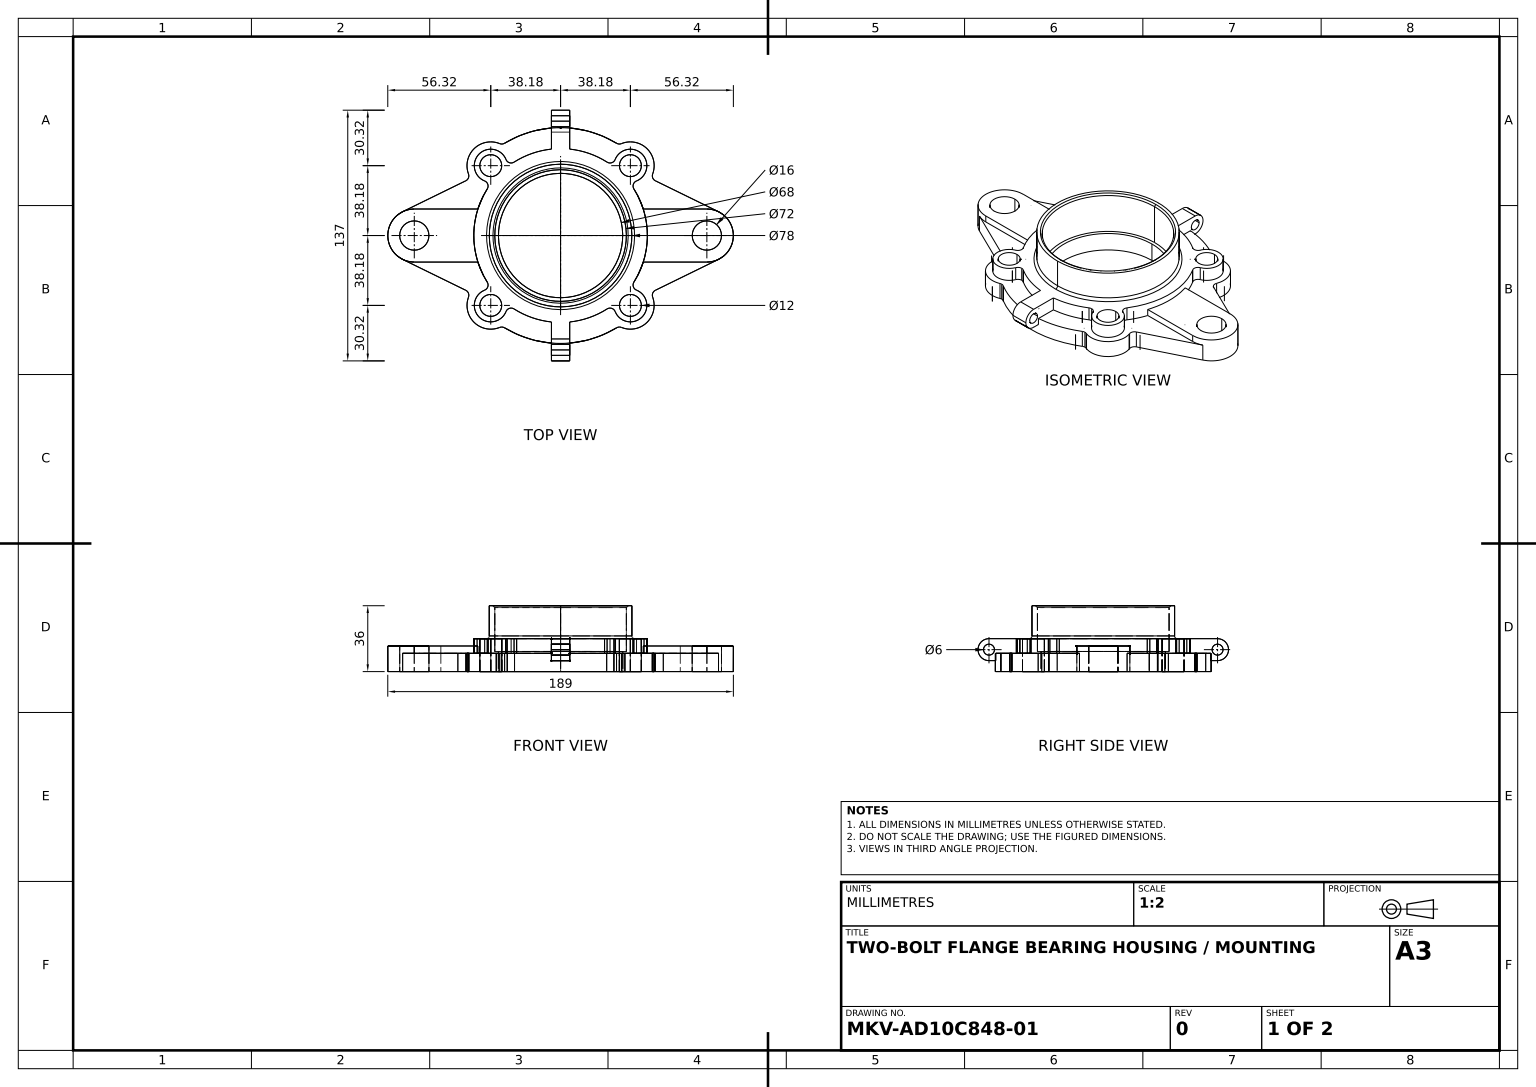
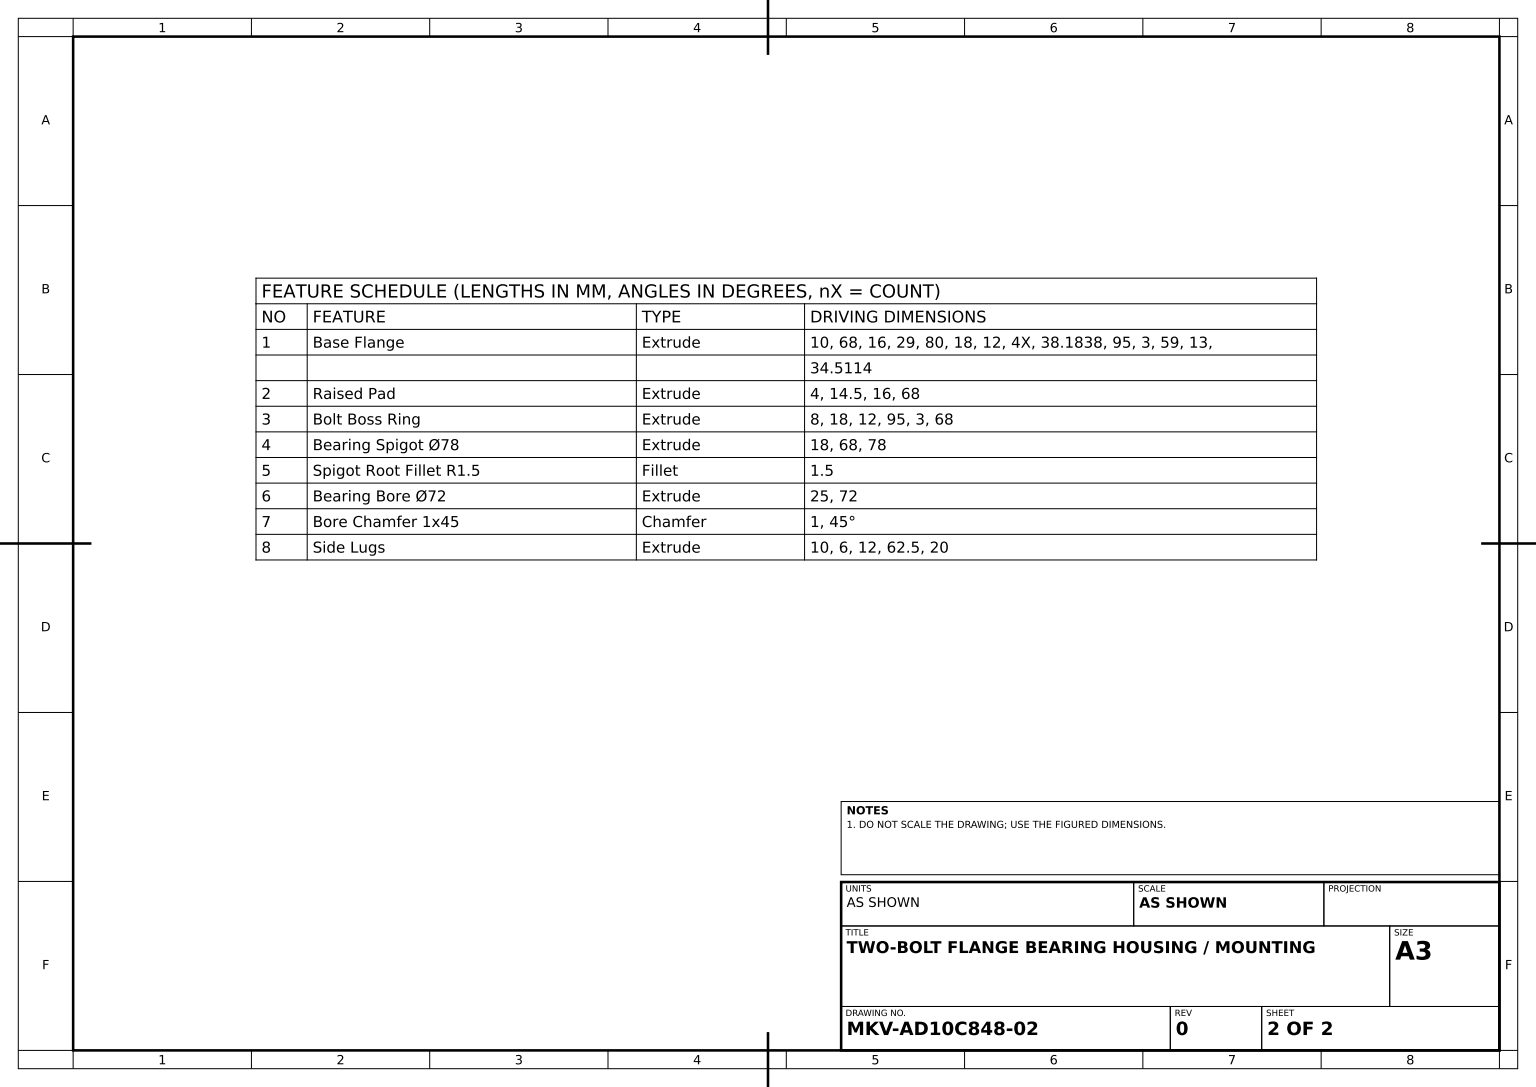
SolidWorks part; units mm, degrees
material "Plain Carbon Steel"
ref_plane "Front Plane" through (0, 0, 0) normal (0, 0, 1) x (1, 0, 0)
ref_plane "Top Plane" through (0, 0, 0) normal (0, 1, 0) x (1, 0, 0)
ref_plane "Right Plane" through (0, 0, 0) normal (1, 0, 0) x (0, 0, -1)
sketch "Base Flange Sketch" plane through (0, 0, 0) normal (0, 1, 0) x (1, 0, 0)
  line L0 (-86.3725, 13.0246) -> (-51.8611, 29.9099)
  line L1 (-86.3725, -13.0246) -> (-51.8611, -29.9099)
  line L2 (86.3725, 13.0246) -> (51.8611, 29.9099)
  line L3 (86.3725, -13.0246) -> (51.8611, -29.9099)
  line L4 (-80, 14.5) -> (-45.2327, 14.5)
  line L5 (-80, -14.5) -> (-45.2327, -14.5)
  line L6 (45.2327, 14.5) -> (80, 14.5)
  line L7 (45.2327, -14.5) -> (80, -14.5)
  circle A0 centre (0, 0) radius 34
  circle A4 centre (-80, 0) radius 8
  arc A5 (-80, 14.5) -> (-80, -14.5) centre (-80, 0) ccw
  arc A6 (80, -14.5) -> (80, 14.5) centre (80, 0) ccw
  circle A7 centre (80, 0) radius 8
  arc A8 (-29.8296, 41.5317) -> (-41.5317, 29.8296) centre (-38.1838, 38.1838) ccw
  circle A10 centre (-38.1838, 38.1838) radius 6
  arc A11 (50.3678, 33.6507) -> (33.2898, 50.2274) centre (38.1838, 38.1838) ccw
  arc A12 (41.5317, 29.8296) -> (29.8296, 41.5317) centre (38.1838, 38.1838) ccw
  circle A13 centre (38.1838, 38.1838) radius 6
  arc A14 (33.2898, -50.2274) -> (50.3678, -33.6507) centre (38.1838, -38.1838) ccw
  arc A15 (29.8296, -41.5317) -> (41.5317, -29.8296) centre (38.1838, -38.1838) ccw
  circle A16 centre (38.1838, -38.1838) radius 6
  arc A17 (-50.3678, -33.6507) -> (-33.2898, -50.2274) centre (-38.1838, -38.1838) ccw
  arc A18 (-41.5317, -29.8296) -> (-29.8296, -41.5317) centre (-38.1838, -38.1838) ccw
  circle A19 centre (-38.1838, -38.1838) radius 6
  arc A20 (-40.1141, 25.4383) -> (-40.1141, -25.4383) centre (0, 0) ccw
  arc A21 (-33.2898, 50.2274) -> (-50.3678, 33.6507) centre (-38.1838, 38.1838) ccw
  arc A22 (-25.4383, -40.1141) -> (25.4383, -40.1141) centre (0, 0) ccw
  arc A23 (-30.6042, -50.4418) -> (30.6042, -50.4418) centre (0, 0) ccw
  arc A24 (25.4383, 40.1141) -> (-25.4383, 40.1141) centre (0, 0) ccw
  arc A25 (30.6042, 50.4418) -> (-30.6042, 50.4418) centre (0, 0) ccw
  arc A26 (40.1141, -25.4383) -> (40.1141, 25.4383) centre (0, 0) ccw
  arc A28 (-30.6042, -50.4418) -> (-33.2898, -50.2274) centre (-32.1604, -53.0067) ccw
  arc A29 (-51.8611, -29.9099) -> (-50.3678, -33.6507) centre (-53.1795, -32.6046) cw
  arc A30 (33.2898, -50.2274) -> (30.6042, -50.4418) centre (32.1604, -53.0067) ccw
  arc A31 (50.3678, -33.6507) -> (51.8611, -29.9099) centre (53.1795, -32.6046) cw
  arc A32 (51.8611, 29.9099) -> (50.3678, 33.6507) centre (53.1795, 32.6046) cw
  arc A33 (33.2898, 50.2274) -> (30.6042, 50.4418) centre (32.1604, 53.0067) cw
  arc A34 (-51.8611, 29.9099) -> (-50.3678, 33.6507) centre (-53.1795, 32.6046) ccw
  arc A35 (-30.6042, 50.4418) -> (-33.2898, 50.2274) centre (-32.1604, 53.0067) cw
  arc A36 (29.8296, -41.5317) -> (25.4383, -40.1141) centre (27.0449, -42.6476) ccw
  arc A37 (41.5317, -29.8296) -> (40.1141, -25.4383) centre (42.6476, -27.0449) cw
  arc A38 (41.5317, 29.8296) -> (40.1141, 25.4383) centre (42.6476, 27.0449) ccw
  arc A39 (29.8296, 41.5317) -> (25.4383, 40.1141) centre (27.0449, 42.6476) cw
  arc A40 (-41.5317, 29.8296) -> (-40.1141, 25.4383) centre (-42.6476, 27.0449) cw
  arc A41 (-41.5317, -29.8296) -> (-40.1141, -25.4383) centre (-42.6476, -27.0449) ccw
  arc A42 (-29.8296, 41.5317) -> (-25.4383, 40.1141) centre (-27.0449, 42.6476) ccw
  arc A43 (-29.8296, -41.5317) -> (-25.4383, -40.1141) centre (-27.0449, -42.6476) cw
  point P41 (49.5957, -31.9573)
  point P46 (31.9573, 49.5957)
  point P55 (37.4544, -29.2134)
  point P60 (29.2134, 37.4544)
  dimension "D1" = 68
  dimension "D3" = 95
  dimension "D4" = 16
  dimension "D5" = 29
  dimension "D6" = 29
  dimension "D7" = 16
  dimension "D8" = 38.1838
  dimension "D11" = 3
  dimension "D12" = 18
  dimension "D13" = 12
  dimension "D20" = 3
  dimension "D21" = 3
  dimension "D22" = 3
  dimension "D23" = 59
  dimension "D24" = 13
  dimension "D25" = 13
  dimension "D26" = 13
  dimension "D27" = 13
  dimension "D9" = 80
  dimension "D10" = 80
  dimension "D15" = 38.1838
  dimension "D16" = 38.1838
  dimension "D17" = 38.1838
  dimension "D18" = 38.1838
  dimension "D19" = 38.1838
  dimension "D28" = 34.5114
  dimension "D29" = 34.5114
  dimension "D30" = 34.5114
  dimension "D31" = 34.5114
  dimension "D14" = 4
extrude "Base Flange" add sketch "Base Flange Sketch" along normal blind 10 contours A20 L4 A5 L5 A4 | A43 A18 A41 A20 L5 A5 L1 A29 A17 A28 A23 A30 A14 A31 L3 A6 L7 A26 A37 A15 A36 A22 | A8 A42 A24 A39 A12 A38 A26 L6 A6 L2 A32 A11 A33 A25 A35 A21 A34 L0 A5 L4 A20 A40 | A26 L7 A6 L6 A7 | A18 A43 A22 A36 A15 A37 A26 A38 A12 A39 A24 A42 A8 A40 A20 A41 A0 A10 A13 A16 A19
sketch "Raised Pad Sketch" plane through (0, 10, 0) normal (0, 1, 0) x (1, 0, 0)
  line L0 (-80, 14.5) -> (-30.753, 14.5)
  line L1 (-30.753, -14.5) -> (-80, -14.5)
  line L2 (80, -14.5) -> (30.753, -14.5)
  line L3 (30.753, 14.5) -> (80, 14.5)
  arc A0 (-30.753, 14.5) -> (-30.753, -14.5) centre (0, 0) ccw
  circle A1 centre (-80, 0) radius 8
  arc A2 (-80, 14.5) -> (-80, -14.5) centre (-80, 0) ccw
  circle A3 centre (80, 0) radius 8
  arc A4 (80, -14.5) -> (80, 14.5) centre (80, 0) ccw
  arc A5 (30.753, -14.5) -> (30.753, 14.5) centre (0, 0) ccw
  dimension "D1" = 14.5
  dimension "D2" = 16
  dimension "D3" = 16
  dimension "D4" = 68
extrude "Raised Pad" add sketch "Raised Pad Sketch" along normal blind 4
sketch "Bolt Boss Ring Sketch" plane through (0, 10, 0) normal (0, 1, 0) x (1, 0, 0)
  circle A1 centre (-38.1838, 38.1838) radius 6
  arc A2 (-29.8296, 41.5317) -> (-41.5317, 29.8296) centre (-38.1838, 38.1838) ccw
  circle A3 centre (38.1838, 38.1838) radius 6
  arc A4 (41.5317, 29.8296) -> (29.8296, 41.5317) centre (38.1838, 38.1838) ccw
  circle A5 centre (38.1838, -38.1838) radius 6
  arc A6 (29.8296, -41.5317) -> (41.5317, -29.8296) centre (38.1838, -38.1838) ccw
  circle A7 centre (-38.1838, -38.1838) radius 6
  arc A8 (-41.5317, -29.8296) -> (-29.8296, -41.5317) centre (-38.1838, -38.1838) ccw
  arc A9 (-40.1141, 25.4383) -> (-40.1141, -25.4383) centre (0, 0) ccw
  arc A10 (25.4383, 40.1141) -> (-25.4383, 40.1141) centre (0, 0) ccw
  arc A11 (-25.4383, -40.1141) -> (25.4383, -40.1141) centre (0, 0) ccw
  arc A12 (40.1141, -25.4383) -> (40.1141, 25.4383) centre (0, 0) ccw
  arc A13 (41.5317, -29.8296) -> (40.1141, -25.4383) centre (42.6476, -27.0449) cw
  arc A14 (29.8296, -41.5317) -> (25.4383, -40.1141) centre (27.0449, -42.6476) ccw
  arc A15 (-41.5317, -29.8296) -> (-40.1141, -25.4383) centre (-42.6476, -27.0449) ccw
  arc A16 (41.5317, 29.8296) -> (40.1141, 25.4383) centre (42.6476, 27.0449) ccw
  arc A17 (29.8296, 41.5317) -> (25.4383, 40.1141) centre (27.0449, 42.6476) cw
  arc A18 (-41.5317, 29.8296) -> (-40.1141, 25.4383) centre (-42.6476, 27.0449) cw
  arc A19 (-29.8296, 41.5317) -> (-25.4383, 40.1141) centre (-27.0449, 42.6476) ccw
  arc A20 (-29.8296, -41.5317) -> (-25.4383, -40.1141) centre (-27.0449, -42.6476) cw
  circle A21 centre (0, 0) radius 34
  point P25 (37.4544, -29.2134)
  point P34 (29.2134, 37.4544)
  dimension "D1" = 18
  dimension "D2" = 12
  dimension "D3" = 12
  dimension "D4" = 18
  dimension "D5" = 12
  dimension "D6" = 12
  dimension "D7" = 18
  dimension "D8" = 18
  dimension "D9" = 95
  dimension "D10" = 3
  dimension "D11" = 3
  dimension "D12" = 3
  dimension "D13" = 68
extrude "Bolt Boss Ring" add sketch "Bolt Boss Ring Sketch" along normal blind 8
sketch "Bearing Spigot Sketch" plane through (0, 18, 0) normal (0, 1, 0) x (1, 0, 0)
  circle A0 centre (0, 0) radius 34
  circle A1 centre (0, 0) radius 39
  dimension "D1" = 68
  dimension "D2" = 78
extrude "Bearing Spigot Ø78" add sketch "Bearing Spigot Sketch" along normal blind 18
fillet "Spigot Root Fillet R1.5" radius 1.5 1 edges at (0, 18, 39)
sketch "Bearing Bore Sketch" plane through (0, 36, 0) normal (0, 1, 0) x (1, 0, 0)
  circle A0 centre (0, 0) radius 36
  dimension "D1" = 72
extrude "Bearing Bore Ø72" cut sketch "Bearing Bore Sketch" against normal blind 25
chamfer "Bore Chamfer 1x45" distance 1 angle 45 1 edges at (0, 36, 36)
ref_plane "Side Lug Plane" through (0, 0, 0) normal (1, 0, 0) x (0, 0, -1)
sketch "Side Lugs Sketch" plane through (0, 0, 0) normal (1, 0, 0) x (0, 0, -1)
  line L4 (-62.5, 18) -> (-42.5, 18)
  line L5 (-42.5, 18) -> (-42.5, 6)
  line L6 (-42.5, 6) -> (-62.5, 6)
  line L7 (62.5, 18) -> (42.5, 18)
  line L8 (47.1838, 18) -> (29.8296, 18) construction
  line L9 (42.5, 18) -> (42.5, 6)
  line L10 (42.5, 6) -> (62.5, 6)
  circle A0 centre (-62.5, 12) radius 3
  arc A1 (-62.5, 18) -> (-62.5, 6) centre (-62.5, 12) ccw
  circle A2 centre (62.5, 12) radius 3
  arc A3 (62.5, 6) -> (62.5, 18) centre (62.5, 12) ccw
  dimension "D1" = 6
  dimension "D2" = 12
  dimension "D3" = 12
  dimension "D4" = 6
  dimension "D5" = 12
  dimension "D6" = 62.5
  dimension "D7" = 62.5
  dimension "D8" = 12
  dimension "D9" = 20
  dimension "D10" = 20
extrude "Side Lugs" add sketch "Side Lugs Sketch" along normal mid plane 10
